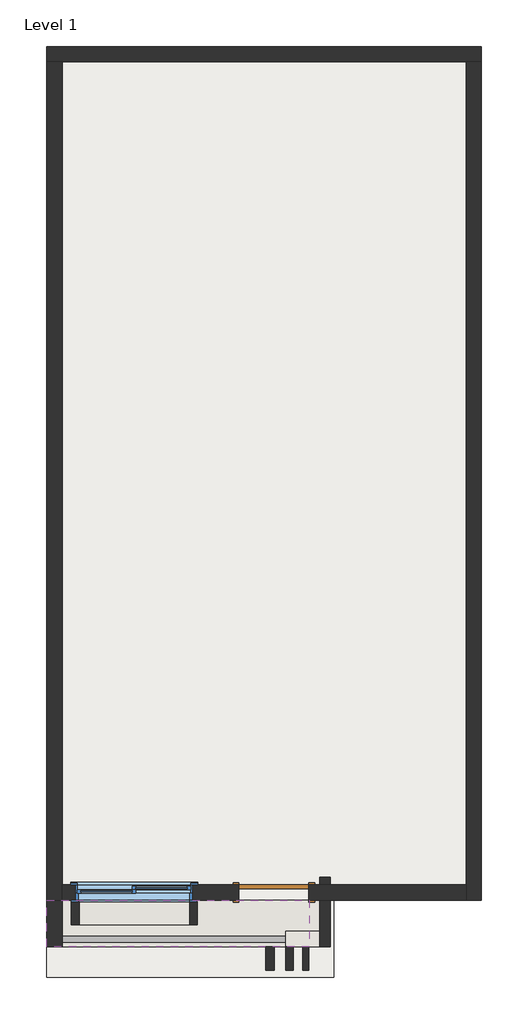
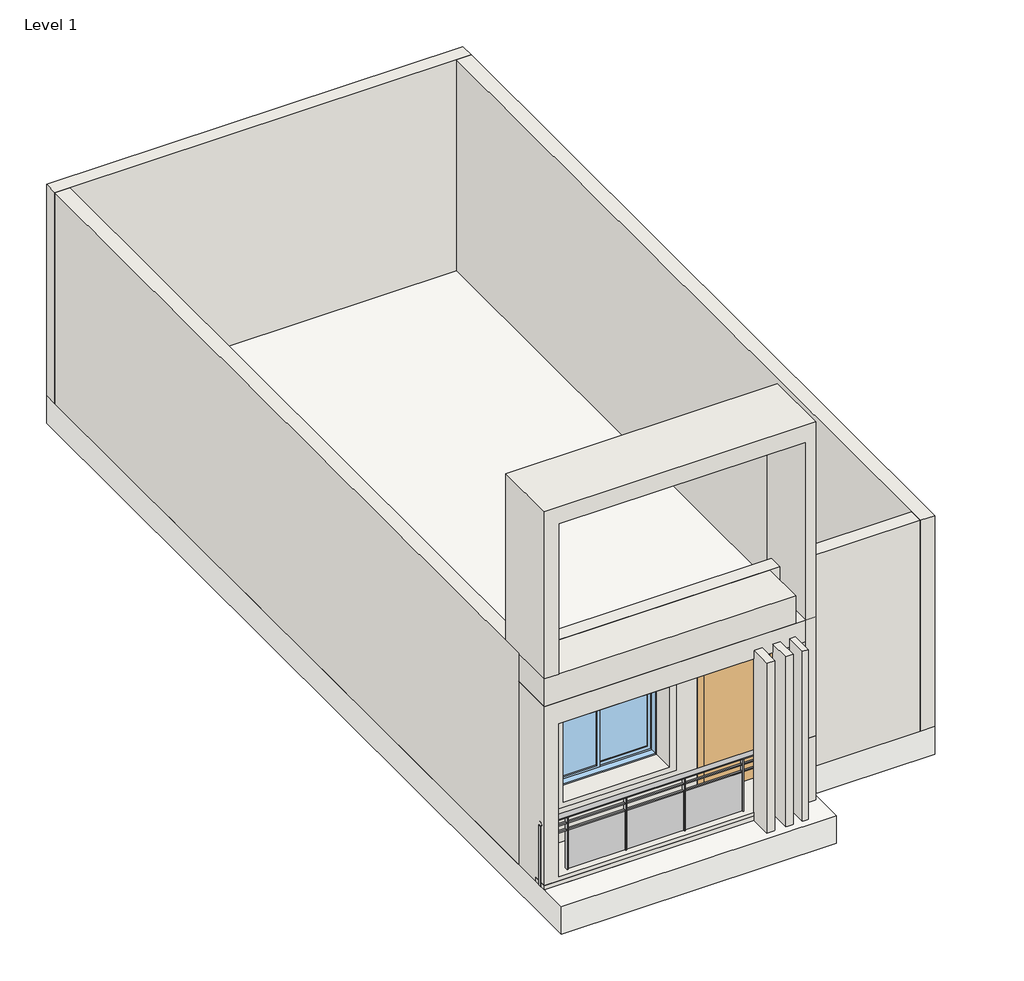
# One storey: 11 walls, 1 door, 1 railing, 1 slab, 1 window.
"""IFC4 building model written with IfcOpenShell, lengths in millimetres."""

from ifc_helpers import new_model, si_unit, point, frame, origin, place, context, project, spatial, polyline, ellipse_curve, trimmed, outline, extrude, faceted_brep, transform, mapped, element, save
from ifc_brep_helpers import plane_surface, extruded_surface, advanced_brep
from components import m_single_flush_0915_x_2134mm_6a9e8738, walls_12_walls_12_7f8ca245, walls_13_walls_13_063eef50, walls_7_walls_7_eccbc88b, walls_8_walls_8_87457aad, walls_9_walls_9_e6c342de, window_c4d7a2b1

model = new_model("IFC4")

# Units and contexts
model_context = context("Model", 3, world=origin())
ifc_project = project(units=[si_unit("LENGTHUNIT", "METRE", prefix="MILLI")], contexts=[model_context])

# Site, building, storey
site = spatial("IfcSite", under=ifc_project)
building = spatial("IfcBuilding", under=site)
storey = spatial("IfcBuildingStorey", under=building, Name="Level 1", Elevation=3048.0)

# Door
placement = place(None, origin())
m_single_flush_0915_x_2134mm_shape = m_single_flush_0915_x_2134mm_6a9e8738(model_context)
element("IfcDoor", 1, ObjectType="M_Single-Flush : 0915 x 2134mm", at=placement, inside=storey, context=model_context, shape_type="MappedRepresentation", body=[
    mapped(m_single_flush_0915_x_2134mm_shape, transform((-6910.1407032, 3960.9956099, 3048.0), x_axis=(1.0, 0.0, 0.0), y_axis=(0.0, 1.0, 0.0), z_axis=(0.0, 0.0, 1.0))),
])

# Railing
element("IfcRailing", 2, ObjectType="Glass Panel - Bottom Fill", at=placement, inside=storey, context=model_context, shape_type="SolidModel", body=[
    advanced_brep(
    [(-9880.3407032, 3390.7863751, 3948.0), (-9880.3407032, 3310.7863751, 3948.0), (-6759.3407032, 3390.7863751, 3948.0), (-6759.3407032, 3310.7863751, 3948.0)],
    [
        (0, 1, ellipse_curve(frame((-9880.3407032, 3350.7863751, 3948.0), z_axis=(-1.0, 0.0, 0.0), x_axis=(0.0, -1.0, 0.0)), 40.0, 30.0)),
        (1, 0, ellipse_curve(frame((-9880.3407032, 3350.7863751, 3948.0), z_axis=(-1.0, 0.0, 0.0), x_axis=(0.0, -1.0, 0.0)), 40.0, 30.0)),
        (2, 3, ellipse_curve(frame((-6759.3407032, 3350.7863751, 3948.0), z_axis=(1.0, 0.0, 0.0), x_axis=(0.0, -1.0, 0.0)), 40.0, 30.0)),
        (3, 2, ellipse_curve(frame((-6759.3407032, 3350.7863751, 3948.0), z_axis=(1.0, 0.0, 0.0), x_axis=(0.0, -1.0, 0.0)), 40.0, 30.0)),
        (0, 2),
        (3, 1),
    ],
    [
        plane_surface(frame((-9880.3407032, 3350.7863751, 3948.0), z_axis=(-1.0, 0.0, 0.0), x_axis=(0.0, 1.0, 0.0))),
        plane_surface(frame((-6759.3407032, 3350.7863751, 3948.0), z_axis=(1.0, 0.0, 0.0), x_axis=(0.0, 1.0, 0.0))),
        extruded_surface(trimmed(ellipse_curve(frame((-6759.3407032, 3350.7863751, 3948.0), z_axis=(-1.0, 0.0, 0.0), x_axis=(0.0, -1.0, 0.0)), 40.0, 30.0), [point((-6759.3407032, 3390.7863751, 3948.0))], [point((-6759.3407032, 3310.7863751, 3948.0))], True, "CARTESIAN"), (-3121.0, 0.0, 0.0), 3121.0),
        extruded_surface(trimmed(ellipse_curve(frame((-6759.3407032, 3350.7863751, 3948.0), z_axis=(-1.0, 0.0, 0.0), x_axis=(0.0, -1.0, 0.0)), 40.0, 30.0), [point((-6759.3407032, 3310.7863751, 3948.0))], [point((-6759.3407032, 3390.7863751, 3948.0))], True, "CARTESIAN"), (-3121.0, 0.0, 0.0), 3121.0),
    ],
    [
        (0, [[1, 2]]),
        (1, [[3, 4]]),
        (2, [[-1, 5, -4, 6]]),
        (3, [[-2, -6, -3, -5]]),
    ],
),
    extrude(outline(polyline([(-9880.3407032, 3341.3956099), (-9880.3407032, 3361.3956099), (-6759.3407032, 3361.3956099), (-6759.3407032, 3341.3956099), (-9880.3407032, 3341.3956099)])), frame((0.0, 0.0, 3828.0), z_axis=(0.0, 0.0, 1.0), x_axis=(1.0, 0.0, 0.0)), (0.0, 0.0, 1.0), 20.0),
    extrude(outline(polyline([(-9880.3407032, 3341.3956099), (-9880.3407032, 3361.3956099), (-6759.3407032, 3361.3956099), (-6759.3407032, 3341.3956099), (-9880.3407032, 3341.3956099)])), frame((0.0, 0.0, 3728.0), z_axis=(0.0, 0.0, 1.0), x_axis=(1.0, 0.0, 0.0)), (0.0, 0.0, 1.0), 20.0),
    extrude(outline(polyline([(-7125.8407032, 3376.3956099), (-7113.8407032, 3376.3956099), (-7113.8407032, 3326.3956099), (-7125.8407032, 3326.3956099), (-7125.8407032, 3376.3956099)])), frame((0.0, 0.0, 3048.0), z_axis=(0.0, 0.0, 1.0), x_axis=(1.0, 0.0, 0.0)), (0.0, 0.0, 1.0), 869.8465326),
    extrude(outline(polyline([(-7919.8407032, 3349.6707998), (-7119.8407032, 3349.6707998), (-7119.8407032, 3344.6707998), (-7919.8407032, 3344.6707998), (-7919.8407032, 3349.6707998)])), frame((0.0, 0.0, 3148.0), z_axis=(0.0, 0.0, 1.0), x_axis=(1.0, 0.0, 0.0)), (0.0, 0.0, 1.0), 580.0),
    extrude(outline(polyline([(-7925.8407032, 3376.3956099), (-7913.8407032, 3376.3956099), (-7913.8407032, 3326.3956099), (-7925.8407032, 3326.3956099), (-7925.8407032, 3376.3956099)])), frame((0.0, 0.0, 3048.0), z_axis=(0.0, 0.0, 1.0), x_axis=(1.0, 0.0, 0.0)), (0.0, 0.0, 1.0), 869.8465326),
    extrude(outline(polyline([(-8719.8407032, 3349.6707998), (-7919.8407032, 3349.6707998), (-7919.8407032, 3344.6707998), (-8719.8407032, 3344.6707998), (-8719.8407032, 3349.6707998)])), frame((0.0, 0.0, 3148.0), z_axis=(0.0, 0.0, 1.0), x_axis=(1.0, 0.0, 0.0)), (0.0, 0.0, 1.0), 580.0),
    extrude(outline(polyline([(-8725.8407032, 3376.3956099), (-8713.8407032, 3376.3956099), (-8713.8407032, 3326.3956099), (-8725.8407032, 3326.3956099), (-8725.8407032, 3376.3956099)])), frame((0.0, 0.0, 3048.0), z_axis=(0.0, 0.0, 1.0), x_axis=(1.0, 0.0, 0.0)), (0.0, 0.0, 1.0), 869.8465326),
    extrude(outline(polyline([(-9519.8407032, 3349.6707998), (-8719.8407032, 3349.6707998), (-8719.8407032, 3344.6707998), (-9519.8407032, 3344.6707998), (-9519.8407032, 3349.6707998)])), frame((0.0, 0.0, 3148.0), z_axis=(0.0, 0.0, 1.0), x_axis=(1.0, 0.0, 0.0)), (0.0, 0.0, 1.0), 580.0),
    extrude(outline(polyline([(-9525.8407032, 3376.3956099), (-9513.8407032, 3376.3956099), (-9513.8407032, 3326.3956099), (-9525.8407032, 3326.3956099), (-9525.8407032, 3376.3956099)])), frame((0.0, 0.0, 3048.0), z_axis=(0.0, 0.0, 1.0), x_axis=(1.0, 0.0, 0.0)), (0.0, 0.0, 1.0), 869.8465326),
    extrude(outline(polyline([(-6767.3407032, 3376.3956099), (-6755.3407032, 3376.3956099), (-6755.3407032, 3326.3956099), (-6767.3407032, 3326.3956099), (-6767.3407032, 3376.3956099)])), frame((0.0, 0.0, 3048.0), z_axis=(0.0, 0.0, 1.0), x_axis=(1.0, 0.0, 0.0)), (0.0, 0.0, 1.0), 869.8465326),
    extrude(outline(polyline([(-9884.3407032, 3376.3956099), (-9872.3407032, 3376.3956099), (-9872.3407032, 3326.3956099), (-9884.3407032, 3326.3956099), (-9884.3407032, 3376.3956099)])), frame((0.0, 0.0, 3048.0), z_axis=(0.0, 0.0, 1.0), x_axis=(1.0, 0.0, 0.0)), (0.0, 0.0, 1.0), 869.8465326),
])

# Slab
element("IfcSlab", 3, ObjectType="Generic Floor - 400mm", at=placement, inside=storey, context=model_context, shape_type="SweptSolid", body=[
    extrude(outline(polyline([(-4193.9407032, 15033.7956099), (-4193.9407032, 3860.9956099), (-6122.7407032, 3860.9956099), (-6122.7407032, 2849.7255409), (-9880.3407032, 2849.7255409), (-9880.3407032, 15033.7956099), (-4193.9407032, 15033.7956099)])), frame((0.0, 0.0, 2648.0), z_axis=(0.0, 0.0, 1.0), x_axis=(1.0, 0.0, 0.0)), (0.0, 0.0, 1.0), 400.0),
])

# Walls
element("IfcWall", 4, ObjectType="Generic - 9\"", at=placement, inside=storey, context=model_context, shape_type="Brep", body=[
    faceted_brep([(-9880.3407032, 14833.7956099, 3048.0), (-9680.3407032, 14833.7956099, 3048.0), (-4393.9407032, 14833.7956099, 3048.0), (-4193.9407032, 14833.7956099, 3048.0), (-4193.9407032, 14833.7956099, 6096.0), (-4393.9407032, 14833.7956099, 6096.0), (-9680.3407032, 14833.7956099, 6096.0), (-9880.3407032, 14833.7956099, 6096.0), (-9880.3407032, 15033.7956099, 3048.0), (-9880.3407032, 15033.7956099, 6096.0), (-4193.9407032, 15033.7956099, 6096.0), (-4193.9407032, 15033.7956099, 3048.0)], [[[0, 1, 2, 3, 4, 5, 6, 7]], [[8, 9, 10, 11]], [[3, 2, 1, 0, 8, 11]], [[7, 6, 5, 4, 10, 9]], [[4, 3, 11, 10]], [[0, 7, 9, 8]]]),
])
element("IfcWall", 5, ObjectType="Generic - 9\"", at=placement, inside=storey, context=model_context, shape_type="Brep", body=[
    faceted_brep([(-4393.9407032, 14833.7956099, 3048.0), (-4393.9407032, 4060.9956099, 3048.0), (-4393.9407032, 3860.9956099, 3048.0), (-4393.9407032, 3860.9956099, 6096.0), (-4393.9407032, 4060.9956099, 6096.0), (-4393.9407032, 14833.7956099, 6096.0), (-4193.9407032, 14833.7956099, 3048.0), (-4193.9407032, 14833.7956099, 6096.0), (-4193.9407032, 3860.9956099, 6096.0), (-4193.9407032, 3860.9956099, 3048.0)], [[[0, 1, 2, 3, 4, 5]], [[6, 7, 8, 9]], [[2, 1, 0, 6, 9]], [[5, 4, 3, 8, 7]], [[0, 5, 7, 6]], [[3, 2, 9, 8]]]),
])
element("IfcWall", 6, ObjectType="Generic - 9\"", at=placement, inside=storey, context=model_context, shape_type="SweptSolid", body=[
    extrude(outline(polyline([(5182.0, -6452.6407032), (3048.0, -6452.6407032), (3048.0, -4393.9407032), (6096.0, -4393.9407032), (6096.0, -9680.3407032), (3048.0, -9680.3407032), (3048.0, -7367.6407032), (5182.0, -7367.6407032), (5182.0, -6452.6407032)]), holes=[polyline([(5181.6, -7976.9407032), (3962.4, -7976.9407032), (3962.4, -9500.9407032), (5181.6, -9500.9407032), (5181.6, -7976.9407032)])]), frame((0.0, 3860.9956099, 0.0), z_axis=(0.0, 1.0, 0.0), x_axis=(0.0, 0.0, 1.0)), (0.0, 0.0, 1.0), 200.0),
])
element("IfcWall", 7, ObjectType="Generic - 9\"", at=placement, inside=storey, context=model_context, shape_type="Brep", body=[
    faceted_brep([(-9680.3407032, 3860.9956099, 3048.0), (-9680.3407032, 4060.9956099, 3048.0), (-9680.3407032, 14833.7956099, 3048.0), (-9680.3407032, 14833.7956099, 6096.0), (-9680.3407032, 4060.9956099, 6096.0), (-9680.3407032, 3860.9956099, 6096.0), (-9880.3407032, 3860.9956099, 3048.0), (-9880.3407032, 3860.9956099, 6096.0), (-9880.3407032, 14833.7956099, 6096.0), (-9880.3407032, 14833.7956099, 3048.0)], [[[0, 1, 2, 3, 4, 5]], [[6, 7, 8, 9]], [[2, 1, 0, 6, 9]], [[5, 4, 3, 8, 7]], [[3, 2, 9, 8]], [[0, 5, 7, 6]]]),
])
element("IfcWall", 8, ObjectType="Generic - 9\"", at=placement, inside=storey, context=model_context, shape_type="Brep", body=[
    faceted_brep([(-6756.1407032, 3251.3956099, 3048.0), (-6171.9407032, 3251.3956099, 3048.0), (-6171.9407032, 3251.3956099, 3977.8300175), (-6756.1407032, 3251.3956099, 3977.8300175), (-6756.1407032, 3251.3956099, 3110.5808036), (-6756.1407032, 3451.3956099, 3048.0), (-6756.1407032, 3451.3956099, 3110.5808036), (-6756.1407032, 3451.3956099, 3977.8300175), (-6171.9407032, 3451.3956099, 3977.8300175), (-6171.9407032, 3451.3956099, 3048.0)], [[[0, 1, 2, 3, 4]], [[5, 6, 7, 8, 9]], [[1, 0, 5, 9]], [[2, 1, 9, 8]], [[3, 2, 8, 7]], [[0, 4, 3, 7, 6, 5]]]),
])
element("IfcWall", 9, ObjectType="Generic - 9\"", at=placement, inside=storey, context=model_context, shape_type="SweptSolid", body=[
    extrude(outline(polyline([(-6756.1407032, 3251.3956099), (-9880.3407032, 3251.3956099), (-9880.3407032, 3451.3956099), (-6756.1407032, 3451.3956099), (-6756.1407032, 3251.3956099)])), frame((0.0, 0.0, 3048.0), z_axis=(0.0, 0.0, 1.0), x_axis=(1.0, 0.0, 0.0)), (0.0, 0.0, 1.0), 62.5808036),
])
walls_12_walls_12_shape = walls_12_walls_12_7f8ca245(model_context)
element("IfcWall", 10, ObjectType="Walls 12 : Walls 12", at=placement, inside=storey, context=model_context, shape_type="MappedRepresentation", body=[
    mapped(walls_12_walls_12_shape, transform((0.0, 0.0, 0.0), x_axis=(1.0, 0.0, 0.0), y_axis=(0.0, 1.0, 0.0), z_axis=(0.0, 0.0, 1.0))),
])
walls_13_walls_13_shape = walls_13_walls_13_063eef50(model_context)
element("IfcWall", 11, ObjectType="Walls 13 : Walls 13", at=placement, inside=storey, context=model_context, shape_type="MappedRepresentation", body=[
    mapped(walls_13_walls_13_shape, transform((0.0, 0.0, 0.0), x_axis=(1.0, 0.0, 0.0), y_axis=(0.0, 1.0, 0.0), z_axis=(0.0, 0.0, 1.0))),
])
walls_7_walls_7_shape = walls_7_walls_7_eccbc88b(model_context)
element("IfcWall", 12, ObjectType="Walls 7 : Walls 7", at=placement, inside=storey, context=model_context, shape_type="MappedRepresentation", body=[
    mapped(walls_7_walls_7_shape, transform((0.0, 0.0, 0.0), x_axis=(1.0, 0.0, 0.0), y_axis=(0.0, 1.0, 0.0), z_axis=(0.0, 0.0, 1.0))),
])
walls_8_walls_8_shape = walls_8_walls_8_87457aad(model_context)
element("IfcWall", 13, ObjectType="Walls 8 : Walls 8", at=placement, inside=storey, context=model_context, shape_type="MappedRepresentation", body=[
    mapped(walls_8_walls_8_shape, transform((0.0, 0.0, 0.0), x_axis=(1.0, 0.0, 0.0), y_axis=(0.0, 1.0, 0.0), z_axis=(0.0, 0.0, 1.0))),
])
walls_9_walls_9_shape = walls_9_walls_9_e6c342de(model_context)
element("IfcWall", 14, ObjectType="Walls 9 : Walls 9", at=placement, inside=storey, context=model_context, shape_type="MappedRepresentation", body=[
    mapped(walls_9_walls_9_shape, transform((0.0, 0.0, 0.0), x_axis=(1.0, 0.0, 0.0), y_axis=(0.0, 1.0, 0.0), z_axis=(0.0, 0.0, 1.0))),
])

# Window
window_shape = window_c4d7a2b1(model_context)
element("IfcWindow", 15, ObjectType="Slider with Trim : 60\" x 48\"", at=placement, inside=storey, context=model_context, shape_type="MappedRepresentation", body=[
    mapped(window_shape, transform((-8738.9407032, 3960.9956099, 3048.0), x_axis=(1.0, 0.0, 0.0), y_axis=(0.0, 1.0, 0.0), z_axis=(0.0, 0.0, 1.0))),
])

save(model, "model.ifc")

# Revit data of these elements
# Type "M_Single-Flush : 0915 x 2134mm"
#   Type Mark = "15"
#   Thickness = 51 mm
#   Height = 2134 mm
#   Trim Projection Ext = 25 mm
#   Trim Projection Int = 25 mm
#   Trim Width = 76 mm
#   Width = 915 mm
#   Door Material = Door - Panel
#   Frame Material = Door - Frame
#   Function = (empty or 0)
#   Wall Closure = (empty or 0)
# Type "Glass Panel - Bottom Fill"
#   built-in parameter 1008612 = 0.019685 (stored number, unit not read)
#   built-in parameter 1008611 = 0.019685 (stored number, unit not read)
#   built-in parameter 1008609 = 0.902231 (stored number, unit not read)
#   built-in parameter 1008604 = 0.19685 (stored number, unit not read)
#   built-in parameter 1008603 = 0.164042 (stored number, unit not read)
#   Railing Height = 900 mm
#   built-in parameter 1008630 = 2
#   built-in parameter 1008610 = 2
# Type "Generic Floor - 400mm"
#   Function = 0
#   Layers, outside or top first: 400 mm no material (function 1)
# Type "Generic - 9\""
#   Layers, outside or top first: 200 mm no material (function 1)
# Type "Slider with Trim : 60\" x 48\""
#   Type Mark = "22"
#   Construction Type Id = "GSP4R"
#   Assembly Code = "B2020100"
#   Analytic Construction = "1/8 in Pilkington single glazing"
#   Visual Light Transmittance = 0.9
#   Solar Heat Gain Coefficient = 0.78
#   Heat Transfer Coefficient (U) = 3.6886 W/(m²·K)
#   Height = 1219.2 mm
#   Default Sill Height = 914.4 mm
#   Trim Projection - Ext. = 19.05 mm
#   Trim Projection - Int. = 19.05 mm
#   Trim Width - Exterior = 88.9 mm
#   Trim Width - Interior = 88.9 mm
#   Width = 1524 mm
#   Window Inset = 19.05 mm
#   Define Thermal Properties by = 1
#   Glass Pane Material = Glass
#   Sash Material = Sash
#   Trim Exterior Material = Trim
#   Trim Interior Material = Trim
#   Wall Closure = (empty or 0)
# Element 1 (IfcDoor, "M_Single-Flush : 0915 x 2134mm")
#   Phase Created = New Construction
#   Materials on its faces: "Door - Frame", "Door - Panel"
# Element 2 (IfcRailing, "Glass Panel - Bottom Fill")
#   Phase Created = New Construction
#   Materials on its faces: "Metal - Stainless Steel,Polished", "Glass"
# Element 3 (IfcSlab, "Generic Floor - 400mm")
#   Height Offset From Level = 0 mm
#   Phase Created = New Construction
#   Materials on its faces: "Default Roof"
# Elements 4, 5, 6, 7 (IfcWall, "Generic - 9\"")
#   Top Offset = 0 mm
#   Base Offset = 0 mm
#   Unconnected Height = 3048 mm
#   wall height = 3048 mm
#   Phase Created = New Construction
#   Base Constraint = Level 1
#   Materials on its faces: "Default Wall"
# Element 8 (IfcWall, "Generic - 9\"")
#   Top Offset = 0 mm
#   Base Offset = 0 mm
#   Unconnected Height = 929.83 mm
#   wall height = 929.83 mm
#   Phase Created = New Construction
#   Base Constraint = Level 1
#   Materials on its faces: "Default Wall"
# Element 9 (IfcWall, "Generic - 9\"")
#   Top Offset = 0 mm
#   Base Offset = 0 mm
#   Unconnected Height = 62.581 mm
#   wall height = 62.581 mm
#   Phase Created = New Construction
#   Base Constraint = Level 1
#   Materials on its faces: "Default Wall"
# Element 10 (IfcWall, "Walls 12 : Walls 12")
#   Phase Created = New Construction
#   Materials on its faces: "Default Wall"
# Element 11 (IfcWall, "Walls 13 : Walls 13")
#   Phase Created = New Construction
#   Materials on its faces: "Default Wall"
# Element 12 (IfcWall, "Walls 7 : Walls 7")
#   Phase Created = New Construction
#   Materials on its faces: "Default Wall"
# Element 13 (IfcWall, "Walls 8 : Walls 8")
#   Phase Created = New Construction
#   Materials on its faces: "Default Wall"
# Element 14 (IfcWall, "Walls 9 : Walls 9")
#   Phase Created = New Construction
#   Materials on its faces: "Default Wall"
# Element 15 (IfcWindow, "Slider with Trim : 60\" x 48\"")
#   Mark = "6"
#   Phase Created = New Construction
#   Materials on its faces: "Sash", "Trim", "Glass"
# Materials
#   "Door - Panel": class "Wood", colour RGB 114 82 51, transparency 0
#   "Door - Frame": colour RGB 153 76 43, transparency 0
#   "Glass": class "Glass", colour RGB 218 227 224, transparency 0.85, Description = "Soda Lime Glass", Cost = 0
#   "Sash": class "Wood", colour RGB 136 99 55, transparency 0
#   "Trim": class "Wood", colour RGB 224 178 126, transparency 0
#   "Metal - Stainless Steel,Polished": class "Metal", colour RGB 189 187 185, transparency 0, Cost = 0
#   "Default Roof": colour RGB 80 80 80, transparency 0
#   "Default Wall": colour RGB 80 80 80, transparency 0
